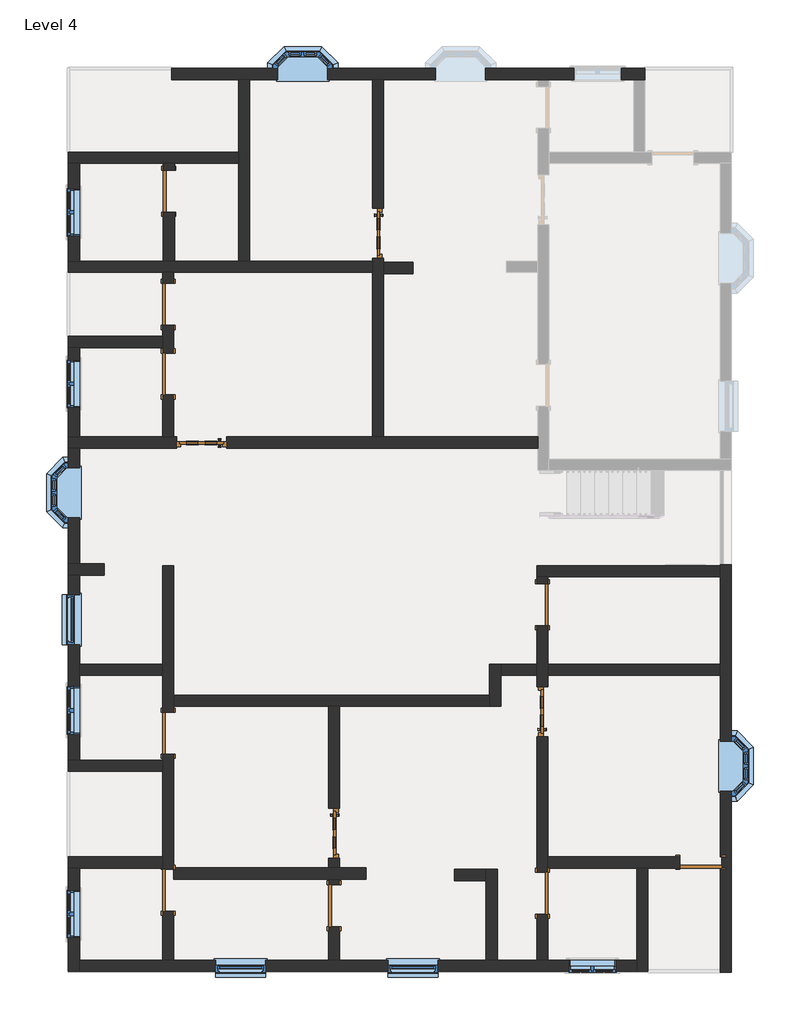
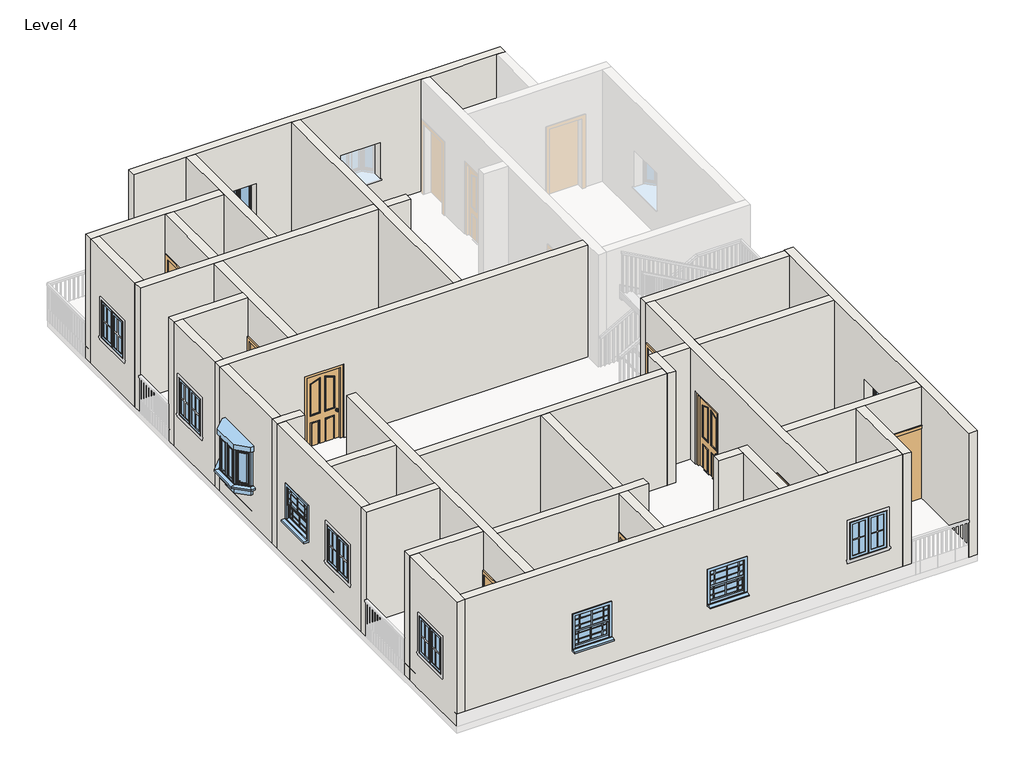
# One storey, part 1 of 4: 34 walls, 13 doors, 11 windows.
"""IFC4 building model written with IfcOpenShell, lengths in millimetres."""

from ifc_helpers import new_model, si_unit, frame, origin, place, context, project, spatial, polyline, outline, extrude, faceted_brep, transform, mapped, element, save
from components import doors_extsgl_12_910x2110mm_9a09825e, door_fadea3f2, door_53b1b562, window_910x910mm_67ef725a, window_c29befe5, windows_sash_w_bars_1_910x910mm_b688f793

model = new_model("IFC4")

# Units and contexts
model_context = context("Model", 3, world=origin())
ifc_project = project(units=[si_unit("LENGTHUNIT", "METRE", prefix="MILLI")], contexts=[model_context])

# Site, building, storey
site = spatial("IfcSite", under=ifc_project)
building = spatial("IfcBuilding", under=site)
storey = spatial("IfcBuildingStorey", under=building, Name="Level 4", Elevation=9144.0)

# Doors
placement = place(None, origin())
doors_extsgl_12_910x2110mm_shape = doors_extsgl_12_910x2110mm_9a09825e(model_context)
element("IfcDoor", 1, ObjectType="Doors_ExtSgl_12 : 910x2110mm", at=placement, inside=storey, context=model_context, shape_type="MappedRepresentation", body=[
    mapped(doors_extsgl_12_910x2110mm_shape, transform((-1409.2058717, 5320.2339901, 9144.0), x_axis=(0.0, -1.0, 0.0), y_axis=(1.0, 0.0, 0.0), z_axis=(0.0, 0.0, 1.0))),
])
element("IfcDoor", 2, ObjectType="Doors_ExtSgl_12 : 910x2110mm", at=placement, inside=storey, context=model_context, shape_type="MappedRepresentation", body=[
    mapped(doors_extsgl_12_910x2110mm_shape, transform((-4622.3058717, 1514.4547293, 9144.0), x_axis=(-1.0, 0.0, 0.0), y_axis=(0.0, -1.0, 0.0), z_axis=(0.0, 0.0, 1.0))),
])
element("IfcDoor", 3, ObjectType="Doors_ExtSgl_12 : 910x2110mm", at=placement, inside=storey, context=model_context, shape_type="MappedRepresentation", body=[
    mapped(doors_extsgl_12_910x2110mm_shape, transform((-2209.3058717, -5597.5452707, 9144.0), x_axis=(0.0, -1.0, 0.0), y_axis=(1.0, 0.0, 0.0), z_axis=(0.0, 0.0, 1.0))),
])
element("IfcDoor", 4, ObjectType="Doors_ExtSgl_12 : 910x2110mm", at=placement, inside=storey, context=model_context, shape_type="MappedRepresentation", body=[
    mapped(doors_extsgl_12_910x2110mm_shape, transform((1587.9941283, -3384.0437545, 9144.0), x_axis=(0.0, 1.0, 0.0), y_axis=(-1.0, 0.0, 0.0), z_axis=(0.0, 0.0, 1.0))),
])
door_shape = door_fadea3f2(model_context)
element("IfcDoor", 5, ObjectType="Single-Flush : 30\" x 80\"", at=placement, inside=storey, context=model_context, shape_type="MappedRepresentation", body=[
    mapped(door_shape, transform((-5219.2058717, 6086.4547293, 9144.0), x_axis=(0.0, 1.0, 0.0), y_axis=(-1.0, 0.0, 0.0), z_axis=(0.0, 0.0, 1.0))),
])
element("IfcDoor", 6, ObjectType="Single-Flush : 30\" x 80\"", at=placement, inside=storey, context=model_context, shape_type="MappedRepresentation", body=[
    mapped(door_shape, transform((-5231.9058717, -6637.2703483, 9144.0), x_axis=(0.0, 1.0, 0.0), y_axis=(-1.0, 0.0, 0.0), z_axis=(0.0, 0.0, 1.0))),
])
element("IfcDoor", 7, ObjectType="Single-Flush : 30\" x 80\"", at=placement, inside=storey, context=model_context, shape_type="MappedRepresentation", body=[
    mapped(door_shape, transform((-2209.3058717, -6918.3452707, 9144.0), x_axis=(0.0, 1.0, 0.0), y_axis=(-1.0, 0.0, 0.0), z_axis=(0.0, 0.0, 1.0))),
])
door_2_shape = door_53b1b562(model_context)
element("IfcDoor", 8, ObjectType="Single-Flush : 30\" x 80\"", at=placement, inside=storey, context=model_context, shape_type="MappedRepresentation", body=[
    mapped(door_2_shape, transform((-5231.9058717, 2759.0547293, 9144.0), x_axis=(0.0, -1.0, 0.0), y_axis=(1.0, 0.0, 0.0), z_axis=(0.0, 0.0, 1.0))),
])
element("IfcDoor", 9, ObjectType="Single-Flush : 30\" x 80\"", at=placement, inside=storey, context=model_context, shape_type="MappedRepresentation", body=[
    mapped(door_2_shape, transform((-5231.9058717, -3778.816952, 9144.0), x_axis=(0.0, -1.0, 0.0), y_axis=(1.0, 0.0, 0.0), z_axis=(0.0, 0.0, 1.0))),
])
element("IfcDoor", 10, ObjectType="Single-Flush : 30\" x 80\"", at=placement, inside=storey, context=model_context, shape_type="MappedRepresentation", body=[
    mapped(door_2_shape, transform((1587.9941283, -6689.7452707, 9144.0), x_axis=(0.0, 1.0, 0.0), y_axis=(-1.0, 0.0, 0.0), z_axis=(0.0, 0.0, 1.0))),
])
element("IfcDoor", 11, ObjectType="Single-Flush : 30\" x 80\"", at=placement, inside=storey, context=model_context, shape_type="MappedRepresentation", body=[
    mapped(door_2_shape, transform((4470.8941283, -6130.9452707, 9144.0), x_axis=(1.0, 0.0, 0.0), y_axis=(0.0, 1.0, 0.0), z_axis=(0.0, 0.0, 1.0))),
])
element("IfcDoor", 12, ObjectType="Single-Flush : 30\" x 80\"", at=placement, inside=storey, context=model_context, shape_type="MappedRepresentation", body=[
    mapped(door_2_shape, transform((1587.9941283, -1440.3867138, 9144.0), x_axis=(0.0, 1.0, 0.0), y_axis=(-1.0, 0.0, 0.0), z_axis=(0.0, 0.0, 1.0))),
])
element("IfcDoor", 13, ObjectType="Single-Flush : 30\" x 80\"", at=placement, inside=storey, context=model_context, shape_type="MappedRepresentation", body=[
    mapped(door_2_shape, transform((-5231.9058717, 4026.9443597, 9144.0), x_axis=(0.0, -1.0, 0.0), y_axis=(1.0, 0.0, 0.0), z_axis=(0.0, 0.0, 1.0))),
])

# Walls
element("IfcWall", 14, ObjectType="Generic - 4.5\"", at=placement, inside=storey, context=model_context, shape_type="Brep", body=[
    faceted_brep([(-1510.8058717, 4865.2339901, 11254.0), (-1510.8058717, 4865.2339901, 9144.0), (-1510.8058717, 4812.2339901, 9144.0), (-1510.8058717, 4609.0339901, 9144.0), (-1510.8058717, 1616.0547293, 9144.0), (-1510.8058717, 1616.0547293, 12192.0), (-1510.8058717, 4609.0339901, 12192.0), (-1510.8058717, 4812.2339901, 12192.0), (-1510.8058717, 8118.4547293, 12192.0), (-1510.8058717, 8118.4547293, 9144.0), (-1510.8058717, 5775.2339901, 9144.0), (-1510.8058717, 5775.2339901, 11254.0), (-1307.6058717, 1616.0547293, 9144.0), (-1307.6058717, 4587.8547293, 9144.0), (-1307.6058717, 4791.0547293, 9144.0), (-1307.6058717, 4865.2339901, 9144.0), (-1307.6058717, 4865.2339901, 11254.0), (-1307.6058717, 5775.2339901, 11254.0), (-1307.6058717, 5775.2339901, 9144.0), (-1307.6058717, 8118.4547293, 9144.0), (-1307.6058717, 8118.4547293, 12192.0), (-1307.6058717, 4791.0547293, 12192.0), (-1307.6058717, 4587.8547293, 12192.0), (-1307.6058717, 1616.0547293, 12192.0)], [[[0, 1, 2, 3, 4, 5, 6, 7, 8, 9, 10, 11]], [[12, 13, 14, 15, 16, 17, 18, 19, 20, 21, 22, 23]], [[10, 9, 19, 18]], [[4, 3, 2, 1, 15, 14, 13, 12]], [[8, 7, 6, 5, 23, 22, 21, 20]], [[9, 8, 20, 19]], [[5, 4, 12, 23]], [[18, 17, 11, 10]], [[16, 15, 1, 0]], [[17, 16, 0, 11]]]),
])
element("IfcWall", 15, ObjectType="Generic - 4.5\"", at=placement, inside=storey, context=model_context, shape_type="Brep", body=[
    faceted_brep([(-7048.0058717, 4609.0339901, 9144.0), (-5333.5058717, 4609.0339901, 9144.0), (-5130.3058717, 4609.0339901, 9144.0), (-1510.8058717, 4609.0339901, 9144.0), (-1510.8058717, 4609.0339901, 12192.0), (-5130.3058717, 4609.0339901, 12192.0), (-5333.5058717, 4609.0339901, 12192.0), (-7048.0058717, 4609.0339901, 12192.0), (-7048.0058717, 4812.2339901, 9144.0), (-7048.0058717, 4812.2339901, 12192.0), (-6844.8058717, 4812.2339901, 12192.0), (-5320.8058717, 4812.2339901, 12192.0), (-5117.6058717, 4812.2339901, 12192.0), (-3949.2058717, 4812.2339901, 12192.0), (-3746.0058717, 4812.2339901, 12192.0), (-1510.8058717, 4812.2339901, 12192.0), (-1510.8058717, 4812.2339901, 9144.0), (-3746.0058717, 4812.2339901, 9144.0), (-3949.2058717, 4812.2339901, 9144.0), (-5117.6058717, 4812.2339901, 9144.0), (-5320.8058717, 4812.2339901, 9144.0), (-6844.8058717, 4812.2339901, 9144.0)], [[[0, 1, 2, 3, 4, 5, 6, 7]], [[8, 9, 10, 11, 12, 13, 14, 15, 16, 17, 18, 19, 20, 21]], [[3, 2, 1, 0, 8, 21, 20, 19, 18, 17, 16]], [[7, 6, 5, 4, 15, 14, 13, 12, 11, 10, 9]], [[4, 3, 16, 15]], [[0, 7, 9, 8]]]),
])
element("IfcWall", 16, ObjectType="Generic - 4.5\"", at=placement, inside=storey, context=model_context, shape_type="Brep", body=[
    faceted_brep([(-3949.2058717, 8118.4547293, 9144.0), (-3949.2058717, 6797.6547293, 9144.0), (-3949.2058717, 6594.4547293, 9144.0), (-3949.2058717, 4812.2339901, 9144.0), (-3949.2058717, 4812.2339901, 12192.0), (-3949.2058717, 6594.4547293, 12192.0), (-3949.2058717, 6797.6547293, 12192.0), (-3949.2058717, 8118.4547293, 12192.0), (-3746.0058717, 8118.4547293, 9144.0), (-3746.0058717, 8118.4547293, 12192.0), (-3746.0058717, 4812.2339901, 12192.0), (-3746.0058717, 4812.2339901, 9144.0)], [[[0, 1, 2, 3, 4, 5, 6, 7]], [[8, 9, 10, 11]], [[3, 2, 1, 0, 8, 11]], [[7, 6, 5, 4, 10, 9]], [[0, 7, 9, 8]], [[4, 3, 11, 10]]]),
])
element("IfcWall", 17, ObjectType="Generic - 4.5\"", at=placement, inside=storey, context=model_context, shape_type="Brep", body=[
    faceted_brep([(-5333.5058717, 3645.9443597, 11176.0), (-5333.5058717, 3645.9443597, 9144.0), (-5333.5058717, 3444.8547293, 9144.0), (-5333.5058717, 3241.6547293, 9144.0), (-5333.5058717, 3140.0547293, 9144.0), (-5333.5058717, 3140.0547293, 11176.0), (-5333.5058717, 2378.0547293, 11176.0), (-5333.5058717, 2378.0547293, 9144.0), (-5333.5058717, 1616.0547293, 9144.0), (-5333.5058717, 1616.0547293, 12192.0), (-5333.5058717, 3241.6547293, 12192.0), (-5333.5058717, 3444.8547293, 12192.0), (-5333.5058717, 4609.0339901, 12192.0), (-5333.5058717, 4609.0339901, 9144.0), (-5333.5058717, 4407.9443597, 9144.0), (-5333.5058717, 4407.9443597, 11176.0), (-5130.3058717, 3140.0547293, 9144.0), (-5130.3058717, 3645.9443597, 9144.0), (-5130.3058717, 3645.9443597, 11176.0), (-5130.3058717, 4407.9443597, 11176.0), (-5130.3058717, 4407.9443597, 9144.0), (-5130.3058717, 4609.0339901, 9144.0), (-5130.3058717, 4609.0339901, 12192.0), (-5130.3058717, 1616.0547293, 12192.0), (-5130.3058717, 1616.0547293, 9144.0), (-5130.3058717, 2378.0547293, 9144.0), (-5130.3058717, 2378.0547293, 11176.0), (-5130.3058717, 3140.0547293, 11176.0)], [[[0, 1, 2, 3, 4, 5, 6, 7, 8, 9, 10, 11, 12, 13, 14, 15]], [[16, 17, 18, 19, 20, 21, 22, 23, 24, 25, 26, 27]], [[8, 7, 25, 24]], [[14, 13, 21, 20]], [[4, 3, 2, 1, 17, 16]], [[12, 11, 10, 9, 23, 22]], [[13, 12, 22, 21]], [[9, 8, 24, 23]], [[26, 25, 7, 6]], [[27, 26, 6, 5]], [[16, 27, 5, 4]], [[18, 17, 1, 0]], [[19, 18, 0, 15]], [[20, 19, 15, 14]]]),
])
element("IfcWall", 18, ObjectType="Generic - 4.5\"", at=placement, inside=storey, context=model_context, shape_type="Brep", body=[
    faceted_brep([(-5130.3058717, -6256.2703483, 11176.0), (-5130.3058717, -6256.2703483, 9144.0), (-5130.3058717, -6230.8703483, 9144.0), (-5130.3058717, -4159.816952, 9144.0), (-5130.3058717, -4159.816952, 11176.0), (-5130.3058717, -3397.816952, 11176.0), (-5130.3058717, -3397.816952, 9144.0), (-5130.3058717, -3286.1452707, 9144.0), (-5130.3058717, -3082.9452707, 9144.0), (-5130.3058717, -733.4452707, 9144.0), (-5130.3058717, -733.4452707, 12192.0), (-5130.3058717, -3082.9452707, 12192.0), (-5130.3058717, -3286.1452707, 12192.0), (-5130.3058717, -6230.8703483, 12192.0), (-5130.3058717, -6434.0703483, 12192.0), (-5130.3058717, -7908.9452707, 12192.0), (-5130.3058717, -7908.9452707, 9144.0), (-5130.3058717, -7018.2703483, 9144.0), (-5130.3058717, -7018.2703483, 11176.0), (-5333.5058717, -4159.816952, 9144.0), (-5333.5058717, -4271.4886333, 9144.0), (-5333.5058717, -4474.6886333, 9144.0), (-5333.5058717, -6029.3452707, 9144.0), (-5333.5058717, -6232.5452707, 9144.0), (-5333.5058717, -6256.2703483, 9144.0), (-5333.5058717, -6256.2703483, 11176.0), (-5333.5058717, -7018.2703483, 11176.0), (-5333.5058717, -7018.2703483, 9144.0), (-5333.5058717, -7908.9452707, 9144.0), (-5333.5058717, -7908.9452707, 12192.0), (-5333.5058717, -6232.5452707, 12192.0), (-5333.5058717, -6029.3452707, 12192.0), (-5333.5058717, -4474.6886333, 12192.0), (-5333.5058717, -4271.4886333, 12192.0), (-5333.5058717, -2727.3452707, 12192.0), (-5333.5058717, -2524.1452707, 12192.0), (-5333.5058717, -733.4452707, 12192.0), (-5333.5058717, -733.4452707, 9144.0), (-5333.5058717, -2524.1452707, 9144.0), (-5333.5058717, -2727.3452707, 9144.0), (-5333.5058717, -3397.816952, 9144.0), (-5333.5058717, -3397.816952, 11176.0), (-5333.5058717, -4159.816952, 11176.0)], [[[0, 1, 2, 3, 4, 5, 6, 7, 8, 9, 10, 11, 12, 13, 14, 15, 16, 17, 18]], [[19, 20, 21, 22, 23, 24, 25, 26, 27, 28, 29, 30, 31, 32, 33, 34, 35, 36, 37, 38, 39, 40, 41, 42]], [[40, 39, 38, 37, 9, 8, 7, 6]], [[17, 16, 28, 27]], [[3, 2, 1, 24, 23, 22, 21, 20, 19]], [[10, 9, 37, 36]], [[15, 14, 13, 12, 11, 10, 36, 35, 34, 33, 32, 31, 30, 29]], [[4, 3, 19, 42]], [[5, 4, 42, 41]], [[6, 5, 41, 40]], [[25, 24, 1, 0]], [[26, 25, 0, 18]], [[27, 26, 18, 17]], [[16, 15, 29, 28]]]),
])
element("IfcWall", 19, ObjectType="Generic - 4.5\"", at=placement, inside=storey, context=model_context, shape_type="Brep", body=[
    faceted_brep([(-7048.0058717, -898.5452707, 9144.0), (-6844.8058717, -898.5452707, 9144.0), (-6400.7404065, -898.5452707, 9144.0), (-6400.7404065, -898.5452707, 12192.0), (-6844.8058717, -898.5452707, 12192.0), (-7048.0058717, -898.5452707, 12192.0), (-7048.0058717, -695.3452707, 9144.0), (-7048.0058717, -695.3452707, 12192.0), (-6844.8058717, -695.3452707, 12192.0), (-6400.7404065, -695.3452707, 12192.0), (-6400.7404065, -695.3452707, 9144.0), (-6844.8058717, -695.3452707, 9144.0)], [[[0, 1, 2, 3, 4, 5]], [[6, 7, 8, 9, 10, 11]], [[2, 1, 0, 6, 11, 10]], [[3, 2, 10, 9]], [[5, 4, 3, 9, 8, 7]], [[0, 5, 7, 6]]]),
])
element("IfcWall", 20, ObjectType="Generic - 4.5\"", at=placement, inside=storey, context=model_context, shape_type="Brep", body=[
    faceted_brep([(-7048.0058717, 6594.4547293, 9144.0), (-6844.8058717, 6594.4547293, 9144.0), (-5320.8058717, 6594.4547293, 9144.0), (-5117.6058717, 6594.4547293, 9144.0), (-3949.2058717, 6594.4547293, 9144.0), (-3949.2058717, 6594.4547293, 12192.0), (-5117.6058717, 6594.4547293, 12192.0), (-5320.8058717, 6594.4547293, 12192.0), (-6844.8058717, 6594.4547293, 12192.0), (-7048.0058717, 6594.4547293, 12192.0), (-7048.0058717, 6797.6547293, 9144.0), (-7048.0058717, 6797.6547293, 12192.0), (-3949.2058717, 6797.6547293, 12192.0), (-3949.2058717, 6797.6547293, 9144.0)], [[[0, 1, 2, 3, 4, 5, 6, 7, 8, 9]], [[10, 11, 12, 13]], [[4, 3, 2, 1, 0, 10, 13]], [[9, 8, 7, 6, 5, 12, 11]], [[5, 4, 13, 12]], [[0, 9, 11, 10]]]),
])
element("IfcWall", 21, ObjectType="Generic - 4.5\"", at=placement, inside=storey, context=model_context, shape_type="Brep", body=[
    faceted_brep([(-7048.0058717, 3241.6547293, 9144.0), (-6844.8058717, 3241.6547293, 9144.0), (-5333.5058717, 3241.6547293, 9144.0), (-5333.5058717, 3241.6547293, 12192.0), (-6844.8058717, 3241.6547293, 12192.0), (-7048.0058717, 3241.6547293, 12192.0), (-7048.0058717, 3444.8547293, 9144.0), (-7048.0058717, 3444.8547293, 12192.0), (-5333.5058717, 3444.8547293, 12192.0), (-5333.5058717, 3444.8547293, 9144.0)], [[[0, 1, 2, 3, 4, 5]], [[6, 7, 8, 9]], [[2, 1, 0, 6, 9]], [[5, 4, 3, 8, 7]], [[3, 2, 9, 8]], [[0, 5, 7, 6]]]),
])
element("IfcWall", 22, ObjectType="Generic - 4.5\"", at=placement, inside=storey, context=model_context, shape_type="Brep", body=[
    faceted_brep([(-7048.0058717, 1412.8547293, 9144.0), (-6844.8058717, 1412.8547293, 9144.0), (-5077.3058717, 1412.8547293, 9144.0), (-5077.3058717, 1412.8547293, 11254.0), (-4167.3058717, 1412.8547293, 11254.0), (-4167.3058717, 1412.8547293, 9144.0), (1499.0941283, 1412.8547293, 9144.0), (1499.0941283, 1412.8547293, 12192.0), (-6844.8058717, 1412.8547293, 12192.0), (-7048.0058717, 1412.8547293, 12192.0), (-5077.3058717, 1616.0547293, 11254.0), (-5077.3058717, 1616.0547293, 9144.0), (-5130.3058717, 1616.0547293, 9144.0), (-5333.5058717, 1616.0547293, 9144.0), (-6844.8058717, 1616.0547293, 9144.0), (-7048.0058717, 1616.0547293, 9144.0), (-7048.0058717, 1616.0547293, 12192.0), (-6844.8058717, 1616.0547293, 12192.0), (-5333.5058717, 1616.0547293, 12192.0), (-5130.3058717, 1616.0547293, 12192.0), (-1510.8058717, 1616.0547293, 12192.0), (-1307.6058717, 1616.0547293, 12192.0), (1499.0941283, 1616.0547293, 12192.0), (1499.0941283, 1616.0547293, 9144.0), (-1307.6058717, 1616.0547293, 9144.0), (-1510.8058717, 1616.0547293, 9144.0), (-4167.3058717, 1616.0547293, 9144.0), (-4167.3058717, 1616.0547293, 11254.0)], [[[0, 1, 2, 3, 4, 5, 6, 7, 8, 9]], [[10, 11, 12, 13, 14, 15, 16, 17, 18, 19, 20, 21, 22, 23, 24, 25, 26, 27]], [[26, 25, 24, 23, 6, 5]], [[15, 14, 13, 12, 11, 2, 1, 0]], [[9, 8, 7, 22, 21, 20, 19, 18, 17, 16]], [[7, 6, 23, 22]], [[5, 4, 27, 26]], [[3, 2, 11, 10]], [[4, 3, 10, 27]], [[0, 9, 16, 15]]]),
])
element("IfcWall", 23, ObjectType="Generic - 4.5\"", at=placement, inside=storey, context=model_context, shape_type="Brep", body=[
    faceted_brep([(1486.3941283, -932.3867138, 9144.0), (1689.5941283, -932.3867138, 9144.0), (4826.4941283, -932.3867138, 9144.0), (4826.4941283, -932.3867138, 12192.0), (1689.5941283, -932.3867138, 12192.0), (1486.3941283, -932.3867138, 12192.0), (1486.3941283, -729.1867138, 9144.0), (1486.3941283, -729.1867138, 12192.0), (4826.4941283, -729.1867138, 12192.0), (4826.4941283, -729.1867138, 9144.0)], [[[0, 1, 2, 3, 4, 5]], [[6, 7, 8, 9]], [[2, 1, 0, 6, 9]], [[5, 4, 3, 8, 7]], [[3, 2, 9, 8]], [[0, 5, 7, 6]]]),
])
element("IfcWall", 24, ObjectType="Generic - 4.5\"", at=placement, inside=storey, context=model_context, shape_type="Brep", body=[
    faceted_brep([(1486.3941283, -932.3867138, 9144.0), (1486.3941283, -1059.3867138, 9144.0), (1486.3941283, -1059.3867138, 11176.0), (1486.3941283, -1821.3867138, 11176.0), (1486.3941283, -1821.3867138, 9144.0), (1486.3941283, -2520.4437545, 9144.0), (1486.3941283, -2723.6437545, 9144.0), (1486.3941283, -2929.0437545, 9144.0), (1486.3941283, -2929.0437545, 11254.0), (1486.3941283, -3839.0437545, 11254.0), (1486.3941283, -3839.0437545, 9144.0), (1486.3941283, -6308.7452707, 9144.0), (1486.3941283, -6308.7452707, 11176.0), (1486.3941283, -7070.7452707, 11176.0), (1486.3941283, -7070.7452707, 9144.0), (1486.3941283, -7908.9452707, 9144.0), (1486.3941283, -7908.9452707, 12192.0), (1486.3941283, -2723.6437545, 12192.0), (1486.3941283, -2520.4437545, 12192.0), (1486.3941283, -932.3867138, 12192.0), (1689.5941283, -1059.3867138, 11176.0), (1689.5941283, -1059.3867138, 9144.0), (1689.5941283, -932.3867138, 9144.0), (1689.5941283, -932.3867138, 12192.0), (1689.5941283, -2520.4437545, 12192.0), (1689.5941283, -2723.6437545, 12192.0), (1689.5941283, -6029.3452707, 12192.0), (1689.5941283, -6232.5452707, 12192.0), (1689.5941283, -7908.9452707, 12192.0), (1689.5941283, -7908.9452707, 9144.0), (1689.5941283, -7070.7452707, 9144.0), (1689.5941283, -7070.7452707, 11176.0), (1689.5941283, -6308.7452707, 11176.0), (1689.5941283, -6308.7452707, 9144.0), (1689.5941283, -6232.5452707, 9144.0), (1689.5941283, -6029.3452707, 9144.0), (1689.5941283, -3839.0437545, 9144.0), (1689.5941283, -3839.0437545, 11254.0), (1689.5941283, -2929.0437545, 11254.0), (1689.5941283, -2929.0437545, 9144.0), (1689.5941283, -2723.6437545, 9144.0), (1689.5941283, -2520.4437545, 9144.0), (1689.5941283, -1821.3867138, 9144.0), (1689.5941283, -1821.3867138, 11176.0)], [[[0, 1, 2, 3, 4, 5, 6, 7, 8, 9, 10, 11, 12, 13, 14, 15, 16, 17, 18, 19]], [[20, 21, 22, 23, 24, 25, 26, 27, 28, 29, 30, 31, 32, 33, 34, 35, 36, 37, 38, 39, 40, 41, 42, 43]], [[30, 29, 15, 14]], [[36, 35, 34, 33, 11, 10]], [[22, 21, 1, 0]], [[42, 41, 40, 39, 7, 6, 5, 4]], [[19, 18, 17, 16, 28, 27, 26, 25, 24, 23]], [[0, 19, 23, 22]], [[10, 9, 37, 36]], [[8, 7, 39, 38]], [[9, 8, 38, 37]], [[12, 11, 33, 32]], [[13, 12, 32, 31]], [[14, 13, 31, 30]], [[2, 1, 21, 20]], [[3, 2, 20, 43]], [[4, 3, 43, 42]], [[16, 15, 29, 28]]]),
])
element("IfcWall", 25, ObjectType="Generic - 4.5\"", at=placement, inside=storey, context=model_context, shape_type="SweptSolid", body=[
    extrude(outline(polyline([(4826.4941283, -2723.6437545), (1689.5941283, -2723.6437545), (1689.5941283, -2520.4437545), (4826.4941283, -2520.4437545), (4826.4941283, -2723.6437545)])), frame((0.0, 0.0, 9144.0), z_axis=(0.0, 0.0, 1.0), x_axis=(1.0, 0.0, 0.0)), (0.0, 0.0, 1.0), 3048.0),
])
element("IfcWall", 26, ObjectType="Generic - 4.5\"", at=placement, inside=storey, context=model_context, shape_type="Brep", body=[
    faceted_brep([(4826.4941283, -6232.5452707, 12192.0), (3505.6941283, -6232.5452707, 12192.0), (3302.4941283, -6232.5452707, 12192.0), (1689.5941283, -6232.5452707, 12192.0), (1689.5941283, -6232.5452707, 9144.0), (3302.4941283, -6232.5452707, 9144.0), (3505.6941283, -6232.5452707, 9144.0), (4089.8941283, -6232.5452707, 9144.0), (4089.8941283, -6232.5452707, 11176.0), (4826.4941283, -6232.5452707, 11176.0), (1689.5941283, -6029.3452707, 12192.0), (4826.4941283, -6029.3452707, 12192.0), (4826.4941283, -6029.3452707, 11176.0), (4089.8941283, -6029.3452707, 11176.0), (4089.8941283, -6029.3452707, 9144.0), (1689.5941283, -6029.3452707, 9144.0)], [[[0, 1, 2, 3, 4, 5, 6, 7, 8, 9]], [[10, 11, 12, 13, 14, 15]], [[4, 15, 14, 7, 6, 5]], [[3, 2, 1, 0, 11, 10]], [[11, 0, 9, 12]], [[4, 3, 10, 15]], [[8, 13, 12, 9]], [[13, 8, 7, 14]]]),
])
element("IfcWall", 27, ObjectType="Generic - 4.5\"", at=placement, inside=storey, context=model_context, shape_type="Brep", body=[
    faceted_brep([(3302.4941283, -6232.5452707, 9144.0), (3302.4941283, -7908.9452707, 9144.0), (3302.4941283, -8112.1452707, 9144.0), (3302.4941283, -8112.1452707, 12192.0), (3302.4941283, -7908.9452707, 12192.0), (3302.4941283, -6232.5452707, 12192.0), (3505.6941283, -6232.5452707, 9144.0), (3505.6941283, -6232.5452707, 12192.0), (3505.6941283, -8112.1452707, 12192.0), (3505.6941283, -8112.1452707, 9144.0)], [[[0, 1, 2, 3, 4, 5]], [[6, 7, 8, 9]], [[2, 1, 0, 6, 9]], [[5, 4, 3, 8, 7]], [[0, 5, 7, 6]], [[3, 2, 9, 8]]]),
])
element("IfcWall", 28, ObjectType="Generic - 4.5\"", at=placement, inside=storey, context=model_context, shape_type="SweptSolid", body=[
    extrude(outline(polyline([(-5333.5058717, -2727.3452707), (-6844.8058717, -2727.3452707), (-6844.8058717, -2524.1452707), (-5333.5058717, -2524.1452707), (-5333.5058717, -2727.3452707)])), frame((0.0, 0.0, 9144.0), z_axis=(0.0, 0.0, 1.0), x_axis=(1.0, 0.0, 0.0)), (0.0, 0.0, 1.0), 3048.0),
])
element("IfcWall", 29, ObjectType="Generic - 4.5\"", at=placement, inside=storey, context=model_context, shape_type="Brep", body=[
    faceted_brep([(-7048.0058717, -4474.6886333, 9144.0), (-5333.5058717, -4474.6886333, 9144.0), (-5333.5058717, -4474.6886333, 12192.0), (-7048.0058717, -4474.6886333, 12192.0), (-7048.0058717, -4271.4886333, 9144.0), (-7048.0058717, -4271.4886333, 12192.0), (-6844.8058717, -4271.4886333, 12192.0), (-5333.5058717, -4271.4886333, 12192.0), (-5333.5058717, -4271.4886333, 9144.0), (-6844.8058717, -4271.4886333, 9144.0)], [[[0, 1, 2, 3]], [[4, 5, 6, 7, 8, 9]], [[1, 0, 4, 9, 8]], [[3, 2, 7, 6, 5]], [[2, 1, 8, 7]], [[0, 3, 5, 4]]]),
])
element("IfcWall", 30, ObjectType="Generic - 4.5\"", at=placement, inside=storey, context=model_context, shape_type="Brep", body=[
    faceted_brep([(-7048.0058717, -6232.5452707, 9144.0), (-6844.8058717, -6232.5452707, 9144.0), (-5333.5058717, -6232.5452707, 9144.0), (-5333.5058717, -6232.5452707, 12192.0), (-6844.8058717, -6232.5452707, 12192.0), (-7048.0058717, -6232.5452707, 12192.0), (-7048.0058717, -6029.3452707, 9144.0), (-7048.0058717, -6029.3452707, 12192.0), (-5333.5058717, -6029.3452707, 12192.0), (-5333.5058717, -6029.3452707, 9144.0)], [[[0, 1, 2, 3, 4, 5]], [[6, 7, 8, 9]], [[2, 1, 0, 6, 9]], [[5, 4, 3, 8, 7]], [[3, 2, 9, 8]], [[0, 5, 7, 6]]]),
])
element("IfcWall", 31, ObjectType="Generic - 4.5\"", at=placement, inside=storey, context=model_context, shape_type="Brep", body=[
    faceted_brep([(-5130.3058717, -6434.0703483, 9144.0), (-2310.9058717, -6434.0703483, 9144.0), (-2107.7058717, -6434.0703483, 9144.0), (-1625.1058717, -6434.0703483, 9144.0), (-1625.1058717, -6434.0703483, 12192.0), (-2107.7058717, -6434.0703483, 12192.0), (-2310.9058717, -6434.0703483, 12192.0), (-5130.3058717, -6434.0703483, 12192.0), (-5130.3058717, -6230.8703483, 9144.0), (-5130.3058717, -6230.8703483, 12192.0), (-2310.9058717, -6230.8703483, 12192.0), (-2107.7058717, -6230.8703483, 12192.0), (-1625.1058717, -6230.8703483, 12192.0), (-1625.1058717, -6230.8703483, 9144.0), (-2107.7058717, -6230.8703483, 9144.0), (-2310.9058717, -6230.8703483, 9144.0), (-5130.3058717, -6256.2703483, 9144.0)], [[[0, 1, 2, 3, 4, 5, 6, 7]], [[8, 9, 10, 11, 12, 13, 14, 15]], [[3, 2, 1, 0, 16, 8, 15, 14, 13]], [[4, 3, 13, 12]], [[7, 6, 5, 4, 12, 11, 10, 9]], [[0, 7, 9, 8, 16]]]),
])
element("IfcWall", 32, ObjectType="Generic - 4.5\"", at=placement, inside=storey, context=model_context, shape_type="Brep", body=[
    faceted_brep([(762.4941283, -7908.9452707, 9144.0), (762.4941283, -6257.9452707, 9144.0), (762.4941283, -6257.9452707, 12192.0), (762.4941283, -7908.9452707, 12192.0), (559.2941283, -7908.9452707, 9144.0), (559.2941283, -7908.9452707, 12192.0), (559.2941283, -6461.1452707, 12192.0), (559.2941283, -6257.9452707, 12192.0), (559.2941283, -6257.9452707, 9144.0), (559.2941283, -6461.1452707, 9144.0)], [[[0, 1, 2, 3]], [[4, 5, 6, 7, 8, 9]], [[1, 0, 4, 9, 8]], [[3, 2, 7, 6, 5]], [[2, 1, 8, 7]], [[0, 3, 5, 4]]]),
])
element("IfcWall", 33, ObjectType="Generic - 4.5\"", at=placement, inside=storey, context=model_context, shape_type="SweptSolid", body=[
    extrude(outline(polyline([(-12.2058717, -6257.9452707), (559.2941283, -6257.9452707), (559.2941283, -6461.1452707), (-12.2058717, -6461.1452707), (-12.2058717, -6257.9452707)])), frame((0.0, 0.0, 9144.0), z_axis=(0.0, 0.0, 1.0), x_axis=(1.0, 0.0, 0.0)), (0.0, 0.0, 1.0), 3048.0),
])
element("IfcWall", 34, ObjectType="Generic - 4.5\"", at=placement, inside=storey, context=model_context, shape_type="SweptSolid", body=[
    extrude(outline(polyline([(-3286.1452707, 12192.0), (-3286.1452707, 9144.0), (-5142.5452707, 9144.0), (-5142.5452707, 11254.0), (-6052.5452707, 11254.0), (-6052.5452707, 9144.0), (-6230.8703483, 9144.0), (-6230.8703483, 12192.0), (-3286.1452707, 12192.0)])), frame((-2310.9058717, 0.0, 0.0), z_axis=(1.0, 0.0, 0.0), x_axis=(0.0, 1.0, 0.0)), (0.0, 0.0, 1.0), 203.2),
    extrude(outline(polyline([(-6537.3452707, 9144.0), (-6537.3452707, 11176.0), (-7299.3452707, 11176.0), (-7299.3452707, 9144.0), (-7908.9452707, 9144.0), (-7908.9452707, 12192.0), (-6434.0703483, 12192.0), (-6434.0703483, 9144.0), (-6537.3452707, 9144.0)])), frame((-2310.9058717, 0.0, 0.0), z_axis=(1.0, 0.0, 0.0), x_axis=(0.0, 1.0, 0.0)), (0.0, 0.0, 1.0), 203.2),
])
element("IfcWall", 35, ObjectType="Generic - 4.5\"", at=placement, inside=storey, context=model_context, shape_type="Brep", body=[
    faceted_brep([(-5130.3058717, -3286.1452707, 9144.0), (-2310.9058717, -3286.1452707, 9144.0), (-2107.7058717, -3286.1452707, 9144.0), (622.0199378, -3286.1452707, 9144.0), (622.0199378, -3286.1452707, 12192.0), (-2107.7058717, -3286.1452707, 12192.0), (-2310.9058717, -3286.1452707, 12192.0), (-5130.3058717, -3286.1452707, 12192.0), (-5130.3058717, -3082.9452707, 9144.0), (-5130.3058717, -3082.9452707, 12192.0), (622.0199378, -3082.9452707, 12192.0), (622.0199378, -3082.9452707, 9144.0)], [[[0, 1, 2, 3, 4, 5, 6, 7]], [[8, 9, 10, 11]], [[3, 2, 1, 0, 8, 11]], [[7, 6, 5, 4, 10, 9]], [[0, 7, 9, 8]], [[4, 3, 11, 10]]]),
])
element("IfcWall", 36, ObjectType="Generic - 4.5\"", at=placement, inside=storey, context=model_context, shape_type="Brep", body=[
    faceted_brep([(825.2199378, -3286.1452707, 9144.0), (825.2199378, -2723.6437545, 9144.0), (825.2199378, -2520.4437545, 9144.0), (825.2199378, -2520.4437545, 12192.0), (825.2199378, -2723.6437545, 12192.0), (825.2199378, -3286.1452707, 12192.0), (622.0199378, -3286.1452707, 9144.0), (622.0199378, -3286.1452707, 12192.0), (622.0199378, -3082.9452707, 12192.0), (622.0199378, -2520.4437545, 12192.0), (622.0199378, -2520.4437545, 9144.0), (622.0199378, -3082.9452707, 9144.0)], [[[0, 1, 2, 3, 4, 5]], [[6, 7, 8, 9, 10, 11]], [[2, 1, 0, 6, 11, 10]], [[5, 4, 3, 9, 8, 7]], [[0, 5, 7, 6]], [[3, 2, 10, 9]]]),
])
element("IfcWall", 37, ObjectType="Generic - 4.5\"", at=placement, inside=storey, context=model_context, shape_type="SweptSolid", body=[
    extrude(outline(polyline([(1486.3941283, -2723.6437545), (825.2199378, -2723.6437545), (825.2199378, -2520.4437545), (1486.3941283, -2520.4437545), (1486.3941283, -2723.6437545)])), frame((0.0, 0.0, 9144.0), z_axis=(0.0, 0.0, 1.0), x_axis=(1.0, 0.0, 0.0)), (0.0, 0.0, 1.0), 3048.0),
])
element("IfcWall", 38, ObjectType="Generic - 4.5\"", at=placement, inside=storey, context=model_context, shape_type="SweptSolid", body=[
    extrude(outline(polyline([(-774.2058717, 4587.8547293), (-1307.6058717, 4587.8547293), (-1307.6058717, 4791.0547293), (-774.2058717, 4791.0547293), (-774.2058717, 4587.8547293)])), frame((0.0, 0.0, 9144.0), z_axis=(0.0, 0.0, 1.0), x_axis=(1.0, 0.0, 0.0)), (0.0, 0.0, 1.0), 3048.0),
])
element("IfcWall", 39, ObjectType="Generic - 4.5\"", at=placement, inside=storey, context=model_context, shape_type="SweptSolid", body=[
    extrude(outline(polyline([(6594.4547293, 9144.0), (6467.4547293, 9144.0), (6467.4547293, 11176.0), (5705.4547293, 11176.0), (5705.4547293, 9144.0), (4812.2339901, 9144.0), (4812.2339901, 12192.0), (6594.4547293, 12192.0), (6594.4547293, 9144.0)])), frame((-5320.8058717, 0.0, 0.0), z_axis=(1.0, 0.0, 0.0), x_axis=(0.0, 1.0, 0.0)), (0.0, 0.0, 1.0), 203.2),
])
element("IfcWall", 40, ObjectType="Generic - 9\"", at=placement, inside=storey, context=model_context, shape_type="Brep", body=[
    faceted_brep([(-5168.4058717, 8118.4547293, 9144.0), (-3949.2058717, 8118.4547293, 9144.0), (-3746.0058717, 8118.4547293, 9144.0), (-1510.8058717, 8118.4547293, 9144.0), (-1307.6058717, 8118.4547293, 9144.0), (1499.0941283, 8118.4547293, 9144.0), (1702.2941283, 8118.4547293, 9144.0), (3251.6941283, 8118.4547293, 9144.0), (3454.8941283, 8118.4547293, 9144.0), (3454.8941283, 8118.4547293, 12192.0), (3251.6941283, 8118.4547293, 12192.0), (1702.2941283, 8118.4547293, 12192.0), (1499.0941283, 8118.4547293, 12192.0), (-1307.6058717, 8118.4547293, 12192.0), (-1510.8058717, 8118.4547293, 12192.0), (-3746.0058717, 8118.4547293, 12192.0), (-3949.2058717, 8118.4547293, 12192.0), (-5168.4058717, 8118.4547293, 12192.0), (-359.2558717, 8118.4547293, 10968.4), (550.7441283, 8118.4547293, 10968.4), (550.7441283, 8118.4547293, 10058.4), (-359.2558717, 8118.4547293, 10058.4), (-3235.8058717, 8118.4547293, 10968.4), (-2325.8058717, 8118.4547293, 10968.4), (-2325.8058717, 8118.4547293, 10058.4), (-3235.8058717, 8118.4547293, 10058.4), (3023.0941283, 8118.4547293, 10972.8), (3023.0941283, 8118.4547293, 10058.4), (2159.4941283, 8118.4547293, 10058.4), (2159.4941283, 8118.4547293, 10972.8), (-5168.4058717, 8321.6547293, 9144.0), (-5168.4058717, 8321.6547293, 12192.0), (3454.8941283, 8321.6547293, 12192.0), (3454.8941283, 8321.6547293, 9144.0), (-359.2558717, 8321.6547293, 10968.4), (-359.2558717, 8321.6547293, 10058.4), (550.7441283, 8321.6547293, 10058.4), (550.7441283, 8321.6547293, 10968.4), (-3235.8058717, 8321.6547293, 10968.4), (-3235.8058717, 8321.6547293, 10058.4), (-2325.8058717, 8321.6547293, 10058.4), (-2325.8058717, 8321.6547293, 10968.4), (3023.0941283, 8321.6547293, 10972.8), (2159.4941283, 8321.6547293, 10972.8), (2159.4941283, 8321.6547293, 10058.4), (3023.0941283, 8321.6547293, 10058.4)], [[[0, 1, 2, 3, 4, 5, 6, 7, 8, 9, 10, 11, 12, 13, 14, 15, 16, 17], [18, 19, 20, 21], [22, 23, 24, 25], [26, 27, 28, 29]], [[30, 31, 32, 33], [34, 35, 36, 37], [38, 39, 40, 41], [42, 43, 44, 45]], [[8, 7, 6, 5, 4, 3, 2, 1, 0, 30, 33]], [[17, 16, 15, 14, 13, 12, 11, 10, 9, 32, 31]], [[0, 17, 31, 30]], [[35, 34, 18, 21]], [[36, 35, 21, 20]], [[37, 36, 20, 19]], [[34, 37, 19, 18]], [[39, 38, 22, 25]], [[40, 39, 25, 24]], [[41, 40, 24, 23]], [[38, 41, 23, 22]], [[27, 26, 42, 45]], [[28, 27, 45, 44]], [[29, 28, 44, 43]], [[26, 29, 43, 42]], [[9, 8, 33, 32]]]),
])
element("IfcWall", 41, ObjectType="Generic - 9\"", at=placement, inside=storey, context=model_context, shape_type="Brep", body=[
    faceted_brep([(4826.4941283, -8124.8452707, 9144.0), (4826.4941283, -8124.8452707, 12192.0), (4826.4941283, -6232.5452707, 12192.0), (4826.4941283, -6029.3452707, 12192.0), (4826.4941283, -2723.6437545, 12192.0), (4826.4941283, -2520.4437545, 12192.0), (4826.4941283, -932.3867138, 12192.0), (4826.4941283, -729.1867138, 12192.0), (4826.4941283, -714.2964201, 12192.0), (4826.4941283, -714.2964201, 9144.0), (4826.4941283, -729.1867138, 9144.0), (4826.4941283, -932.3867138, 9144.0), (4826.4941283, -2520.4437545, 9144.0), (4826.4941283, -2723.6437545, 9144.0), (4826.4941283, -6029.3452707, 9144.0), (4826.4941283, -6029.3452707, 11176.0), (4826.4941283, -6232.5452707, 11176.0), (4826.4941283, -6232.5452707, 9144.0), (4826.4941283, -3921.4945126, 10968.4), (4826.4941283, -4831.4945126, 10968.4), (4826.4941283, -4831.4945126, 10058.4), (4826.4941283, -3921.4945126, 10058.4), (5029.6941283, -8124.8452707, 9144.0), (5029.6941283, -714.2964201, 9144.0), (5029.6941283, -714.2964201, 12192.0), (5029.6941283, -8124.8452707, 12192.0), (5029.6941283, -3921.4945126, 10968.4), (5029.6941283, -3921.4945126, 10058.4), (5029.6941283, -4831.4945126, 10058.4), (5029.6941283, -4831.4945126, 10968.4), (4851.8941283, -6232.5452707, 9144.0), (4851.8941283, -6029.3452707, 9144.0), (4851.8941283, -6232.5452707, 11176.0), (4851.8941283, -6029.3452707, 11176.0)], [[[0, 1, 2, 3, 4, 5, 6, 7, 8, 9, 10, 11, 12, 13, 14, 15, 16, 17], [18, 19, 20, 21]], [[22, 23, 24, 25], [26, 27, 28, 29]], [[23, 22, 0, 17, 30, 31, 14, 13, 12, 11, 10, 9]], [[1, 0, 22, 25]], [[8, 7, 6, 5, 4, 3, 2, 1, 25, 24]], [[9, 8, 24, 23]], [[32, 30, 17, 16]], [[31, 33, 15, 14]], [[33, 32, 16, 15]], [[30, 32, 33, 31]], [[27, 26, 18, 21]], [[28, 27, 21, 20]], [[29, 28, 20, 19]], [[26, 29, 19, 18]]]),
])
element("IfcWall", 42, ObjectType="Generic - 9\"", at=placement, inside=storey, context=model_context, shape_type="SweptSolid", body=[
    extrude(outline(polyline([(6594.4547293, 9144.0), (4812.2339901, 9144.0), (4812.2339901, 12192.0), (6594.4547293, 12192.0), (6594.4547293, 9144.0)]), holes=[polyline([(6135.1443597, 10972.8), (5271.5443597, 10972.8), (5271.5443597, 10058.4), (6135.1443597, 10058.4), (6135.1443597, 10972.8)])]), frame((-7048.0058717, 0.0, 0.0), z_axis=(1.0, 0.0, 0.0), x_axis=(0.0, 1.0, 0.0)), (0.0, 0.0, 1.0), 203.2),
])
element("IfcWall", 43, ObjectType="Generic - 9\"", at=placement, inside=storey, context=model_context, shape_type="SweptSolid", body=[
    extrude(outline(polyline([(3241.6547293, 9144.0), (1616.0547293, 9144.0), (1616.0547293, 12192.0), (3241.6547293, 12192.0), (3241.6547293, 9144.0)]), holes=[polyline([(3013.0547293, 10972.8), (2149.4547293, 10972.8), (2149.4547293, 10058.4), (3013.0547293, 10058.4), (3013.0547293, 10972.8)])]), frame((-7048.0058717, 0.0, 0.0), z_axis=(1.0, 0.0, 0.0), x_axis=(0.0, 1.0, 0.0)), (0.0, 0.0, 1.0), 203.2),
])
element("IfcWall", 44, ObjectType="Generic - 9\"", at=placement, inside=storey, context=model_context, shape_type="Brep", body=[
    faceted_brep([(-7048.0058717, -898.5452707, 9144.0), (-7048.0058717, -4271.4886333, 9144.0), (-7048.0058717, -4271.4886333, 12192.0), (-7048.0058717, -898.5452707, 12192.0), (-7048.0058717, -2166.3452707, 10058.4), (-7048.0058717, -1256.3452707, 10058.4), (-7048.0058717, -1256.3452707, 10968.4), (-7048.0058717, -2166.3452707, 10968.4), (-7048.0058717, -2930.5452707, 10972.8), (-7048.0058717, -3794.1452707, 10972.8), (-7048.0058717, -3794.1452707, 10058.4), (-7048.0058717, -2930.5452707, 10058.4), (-6844.8058717, -898.5452707, 9144.0), (-6844.8058717, -898.5452707, 12192.0), (-6844.8058717, -2524.1452707, 12192.0), (-6844.8058717, -2727.3452707, 12192.0), (-6844.8058717, -4271.4886333, 12192.0), (-6844.8058717, -4271.4886333, 9144.0), (-6844.8058717, -2727.3452707, 9144.0), (-6844.8058717, -2524.1452707, 9144.0), (-6844.8058717, -2166.3452707, 10058.4), (-6844.8058717, -2166.3452707, 10968.4), (-6844.8058717, -1256.3452707, 10968.4), (-6844.8058717, -1256.3452707, 10058.4), (-6844.8058717, -2930.5452707, 10972.8), (-6844.8058717, -2930.5452707, 10058.4), (-6844.8058717, -3794.1452707, 10058.4), (-6844.8058717, -3794.1452707, 10972.8)], [[[0, 1, 2, 3], [4, 5, 6, 7], [8, 9, 10, 11]], [[12, 13, 14, 15, 16, 17, 18, 19], [20, 21, 22, 23], [24, 25, 26, 27]], [[1, 0, 12, 19, 18, 17]], [[3, 2, 16, 15, 14, 13]], [[0, 3, 13, 12]], [[2, 1, 17, 16]], [[21, 20, 4, 7]], [[22, 21, 7, 6]], [[23, 22, 6, 5]], [[20, 23, 5, 4]], [[25, 24, 8, 11]], [[26, 25, 11, 10]], [[27, 26, 10, 9]], [[24, 27, 9, 8]]]),
])
element("IfcWall", 45, ObjectType="Generic - 9\"", at=placement, inside=storey, context=model_context, shape_type="Brep", body=[
    faceted_brep([(-7048.0058717, -6232.5452707, 9144.0), (-7048.0058717, -8112.1452707, 9144.0), (-7048.0058717, -8112.1452707, 12192.0), (-7048.0058717, -6232.5452707, 12192.0), (-7048.0058717, -6638.9452707, 10972.8), (-7048.0058717, -7502.5452707, 10972.8), (-7048.0058717, -7502.5452707, 10058.4), (-7048.0058717, -6638.9452707, 10058.4), (-6844.8058717, -6232.5452707, 9144.0), (-6844.8058717, -6232.5452707, 12192.0), (-6844.8058717, -7908.9452707, 12192.0), (-6844.8058717, -8112.1452707, 12192.0), (-6844.8058717, -8112.1452707, 9144.0), (-6844.8058717, -7908.9452707, 9144.0), (-6844.8058717, -6638.9452707, 10972.8), (-6844.8058717, -6638.9452707, 10058.4), (-6844.8058717, -7502.5452707, 10058.4), (-6844.8058717, -7502.5452707, 10972.8)], [[[0, 1, 2, 3], [4, 5, 6, 7]], [[8, 9, 10, 11, 12, 13], [14, 15, 16, 17]], [[1, 0, 8, 13, 12]], [[3, 2, 11, 10, 9]], [[0, 3, 9, 8]], [[2, 1, 12, 11]], [[15, 14, 4, 7]], [[16, 15, 7, 6]], [[17, 16, 6, 5]], [[14, 17, 5, 4]]]),
])
element("IfcWall", 46, ObjectType="Generic - 9\"", at=placement, inside=storey, context=model_context, shape_type="Brep", body=[
    faceted_brep([(-6844.8058717, -8112.1452707, 9144.0), (3302.4941283, -8112.1452707, 9144.0), (3302.4941283, -8112.1452707, 12192.0), (-6844.8058717, -8112.1452707, 12192.0), (-3456.1058717, -8112.1452707, 10058.4), (-4366.1058717, -8112.1452707, 10058.4), (-4366.1058717, -8112.1452707, 10968.4), (-3456.1058717, -8112.1452707, 10968.4), (-319.2058717, -8112.1452707, 10058.4), (-1229.2058717, -8112.1452707, 10058.4), (-1229.2058717, -8112.1452707, 10968.4), (-319.2058717, -8112.1452707, 10968.4), (2064.2441283, -8112.1452707, 10972.8), (2927.8441283, -8112.1452707, 10972.8), (2927.8441283, -8112.1452707, 10058.4), (2064.2441283, -8112.1452707, 10058.4), (-6844.8058717, -7908.9452707, 9144.0), (-6844.8058717, -7908.9452707, 12192.0), (-5333.5058717, -7908.9452707, 12192.0), (-5130.3058717, -7908.9452707, 12192.0), (-2310.9058717, -7908.9452707, 12192.0), (-2107.7058717, -7908.9452707, 12192.0), (559.2941283, -7908.9452707, 12192.0), (762.4941283, -7908.9452707, 12192.0), (1486.3941283, -7908.9452707, 12192.0), (1689.5941283, -7908.9452707, 12192.0), (3302.4941283, -7908.9452707, 12192.0), (3302.4941283, -7908.9452707, 9144.0), (1689.5941283, -7908.9452707, 9144.0), (1486.3941283, -7908.9452707, 9144.0), (762.4941283, -7908.9452707, 9144.0), (559.2941283, -7908.9452707, 9144.0), (-2107.7058717, -7908.9452707, 9144.0), (-2310.9058717, -7908.9452707, 9144.0), (-5130.3058717, -7908.9452707, 9144.0), (-5333.5058717, -7908.9452707, 9144.0), (-3456.1058717, -7908.9452707, 10058.4), (-3456.1058717, -7908.9452707, 10968.4), (-4366.1058717, -7908.9452707, 10968.4), (-4366.1058717, -7908.9452707, 10058.4), (-319.2058717, -7908.9452707, 10058.4), (-319.2058717, -7908.9452707, 10968.4), (-1229.2058717, -7908.9452707, 10968.4), (-1229.2058717, -7908.9452707, 10058.4), (2064.2441283, -7908.9452707, 10972.8), (2064.2441283, -7908.9452707, 10058.4), (2927.8441283, -7908.9452707, 10058.4), (2927.8441283, -7908.9452707, 10972.8)], [[[0, 1, 2, 3], [4, 5, 6, 7], [8, 9, 10, 11], [12, 13, 14, 15]], [[16, 17, 18, 19, 20, 21, 22, 23, 24, 25, 26, 27, 28, 29, 30, 31, 32, 33, 34, 35], [36, 37, 38, 39], [40, 41, 42, 43], [44, 45, 46, 47]], [[1, 0, 16, 35, 34, 33, 32, 31, 30, 29, 28, 27]], [[3, 2, 26, 25, 24, 23, 22, 21, 20, 19, 18, 17]], [[2, 1, 27, 26]], [[0, 3, 17, 16]], [[37, 36, 4, 7]], [[38, 37, 7, 6]], [[39, 38, 6, 5]], [[36, 39, 5, 4]], [[41, 40, 8, 11]], [[42, 41, 11, 10]], [[43, 42, 10, 9]], [[40, 43, 9, 8]], [[45, 44, 12, 15]], [[46, 45, 15, 14]], [[47, 46, 14, 13]], [[44, 47, 13, 12]]]),
])
element("IfcWall", 47, ObjectType="Generic - 9\"", at=placement, inside=storey, context=model_context, shape_type="SweptSolid", body=[
    extrude(outline(polyline([(1412.8547293, 9144.0), (-695.3452707, 9144.0), (-695.3452707, 12192.0), (1412.8547293, 12192.0), (1412.8547293, 9144.0)]), holes=[polyline([(145.0547293, 10968.4), (145.0547293, 10058.4), (1055.0547293, 10058.4), (1055.0547293, 10968.4), (145.0547293, 10968.4)])]), frame((-7048.0058717, 0.0, 0.0), z_axis=(1.0, 0.0, 0.0), x_axis=(0.0, 1.0, 0.0)), (0.0, 0.0, 1.0), 203.2),
])

# Windows
window_910x910mm_shape = window_910x910mm_67ef725a(model_context)
element("IfcWindow", 48, ObjectType="910x910mm", at=placement, inside=storey, context=model_context, shape_type="MappedRepresentation", body=[
    mapped(window_910x910mm_shape, transform((4919.6375605, -4946.4945126, 8858.4), x_axis=(0.0, -1.0, 0.0), y_axis=(1.0, 0.0, 0.0), z_axis=(0.0, 0.0, 1.0))),
])
element("IfcWindow", 49, ObjectType="910x910mm", at=placement, inside=storey, context=model_context, shape_type="MappedRepresentation", body=[
    mapped(window_910x910mm_shape, transform((-2210.8058717, 8211.5981615, 8858.4), x_axis=(1.0, 0.0, 0.0), y_axis=(0.0, 1.0, 0.0), z_axis=(0.0, 0.0, 1.0))),
])
element("IfcWindow", 50, ObjectType="910x910mm", at=placement, inside=storey, context=model_context, shape_type="MappedRepresentation", body=[
    mapped(window_910x910mm_shape, transform((-6937.9493039, 1170.0547293, 8858.4), x_axis=(0.0, 1.0, 0.0), y_axis=(-1.0, 0.0, 0.0), z_axis=(0.0, 0.0, 1.0))),
])
window_shape = window_c29befe5(model_context)
element("IfcWindow", 51, ObjectType="Window-Casement-Double : 34\" x 36\"", at=placement, inside=storey, context=model_context, shape_type="MappedRepresentation", body=[
    mapped(window_shape, transform((-6946.4058717, 5703.3443597, 9144.0), x_axis=(0.0, 1.0, 0.0), y_axis=(-1.0, 0.0, 0.0), z_axis=(0.0, 0.0, 1.0))),
])
element("IfcWindow", 52, ObjectType="Window-Casement-Double : 34\" x 36\"", at=placement, inside=storey, context=model_context, shape_type="MappedRepresentation", body=[
    mapped(window_shape, transform((-6946.4058717, 2581.2547293, 9144.0), x_axis=(0.0, 1.0, 0.0), y_axis=(-1.0, 0.0, 0.0), z_axis=(0.0, 0.0, 1.0))),
])
element("IfcWindow", 53, ObjectType="Window-Casement-Double : 34\" x 36\"", at=placement, inside=storey, context=model_context, shape_type="MappedRepresentation", body=[
    mapped(window_shape, transform((2496.0441283, -8010.5452707, 9144.0), x_axis=(-1.0, 0.0, 0.0), y_axis=(0.0, -1.0, 0.0), z_axis=(0.0, 0.0, 1.0))),
])
element("IfcWindow", 54, ObjectType="Window-Casement-Double : 34\" x 36\"", at=placement, inside=storey, context=model_context, shape_type="MappedRepresentation", body=[
    mapped(window_shape, transform((-6946.4058717, -7070.7452707, 9144.0), x_axis=(0.0, 1.0, 0.0), y_axis=(-1.0, 0.0, 0.0), z_axis=(0.0, 0.0, 1.0))),
])
element("IfcWindow", 55, ObjectType="Window-Casement-Double : 34\" x 36\"", at=placement, inside=storey, context=model_context, shape_type="MappedRepresentation", body=[
    mapped(window_shape, transform((-6946.4058717, -3362.3452707, 9144.0), x_axis=(0.0, 1.0, 0.0), y_axis=(-1.0, 0.0, 0.0), z_axis=(0.0, 0.0, 1.0))),
])
windows_sash_w_bars_1_910x910mm_shape = windows_sash_w_bars_1_910x910mm_b688f793(model_context)
element("IfcWindow", 56, ObjectType="Windows_Sash_w-Bars_1 : 910x910mm", at=placement, inside=storey, context=model_context, shape_type="MappedRepresentation", body=[
    mapped(windows_sash_w_bars_1_910x910mm_shape, transform((-3911.1058717, -8010.5452707, 9258.4), x_axis=(-1.0, 0.0, 0.0), y_axis=(0.0, -1.0, 0.0), z_axis=(0.0, 0.0, 1.0))),
])
element("IfcWindow", 57, ObjectType="Windows_Sash_w-Bars_1 : 910x910mm", at=placement, inside=storey, context=model_context, shape_type="MappedRepresentation", body=[
    mapped(windows_sash_w_bars_1_910x910mm_shape, transform((-6946.4058717, -1711.3452707, 9258.4), x_axis=(0.0, 1.0, 0.0), y_axis=(-1.0, 0.0, 0.0), z_axis=(0.0, 0.0, 1.0))),
])
element("IfcWindow", 58, ObjectType="Windows_Sash_w-Bars_1 : 910x910mm", at=placement, inside=storey, context=model_context, shape_type="MappedRepresentation", body=[
    mapped(windows_sash_w_bars_1_910x910mm_shape, transform((-774.2058717, -8010.5452707, 9258.4), x_axis=(-1.0, 0.0, 0.0), y_axis=(0.0, -1.0, 0.0), z_axis=(0.0, 0.0, 1.0))),
])

save(model, "model.ifc")

# Revit data of these elements
# Type "Doors_ExtSgl_12 : 910x2110mm"
#   Type Mark = "10"
#   Type Comments = "External Single"
#   Operation = "SingleSwingRight"
#   Construction Type Id = "SGL"
#   Keynote = "L20"
#   Analytic Construction = "Large single-glazed windows"
#   Wrap Layers (Int) from Ext = 0' - 6.98819"
#   Wrap Layers (Ext) from Ext = 0' - 4.03543"
#   Visual Light Transmittance = 0.9
#   Thickness = 0' - 1.73228"
#   Stile Top of Lock rail = 3' - 3.37008"
#   Stile Top Rail = 0' - 5.90551"
#   Stile Shutting = 0' - 4.92126"
#   Stile Muntin Rail = 0' - 4.92126"
#   Stile Lock Rail = 0' - 6.88976"
#   Stile Hanging = 0' - 4.92126"
#   Stile Bottom Rail = 0' - 6.88976"
#   Solar Heat Gain Coefficient = 0.86
#   Rough Width = 2' - 11.82677"
#   Rough Height = 6' - 11.07087"
#   O/A Frame Width = 0' - 2.51969"
#   Heat Transfer Coefficient (U) = 0.979472 BTU/(h·ft²·°F)
#   Handle Z Distance = 3' - 3.37008"
#   Glazing Thickness = 0' - 0.94488"
#   FrameWidth = 0' - 1.65354"
#   FrameOffset - External = 0' - 0.98425"
#   FrameDepth = 0' - 3.50394"
#   Door Panel Width = 2' - 7.77165"
#   Door Panel Thickness = 0' - 1.73228"
#   Door Panel Height = 6' - 6.74016"
#   Cill Thickness = 0' - 2.14567"
#   Cill Projection = 0' - 1.1811"
#   Handle X Distance = 0' - 2.95276"
#   Height = 6' - 11.07087"
#   Structural Tolerance = 0' - 0.25591"
#   Tolerance = 0' - 0.11811"
#   Undercut = 0' - 0.15748"
#   Width = 2' - 11.82677"
#   Cill Extension = 0' - 0.98425"
#   Cavity Closer Width = 0' - 1.9685"
#   Cavity Closer Offset from Ext = 0' - 4.03543"
#   Cavity Closer Depth = 0' - 3.34646"
#   Vis - Ironmongery = yes
#   Vis - Cavity Closers = yes
#   Define Thermal Properties by = 1
#   Function = 1
#   Material Glass = Door - Glazing
#   Material Door = Door - Panel
#   Material Frame = Door - Frame/Mullion
#   Material Ironmongery = Door - Handle
#   Wall Closure = (empty or 0)
# Type "Single-Flush : 30\" x 80\""
#   Type Mark = "5"
#   Construction Type Id = "MDOOR"
#   Assembly Code = "C1020"
#   Analytic Construction = "Metal"
#   Thickness = 0' - 2"
#   Heat Transfer Coefficient (U) = 0.651978 BTU/(h·ft²·°F)
#   Height = 6' - 8"
#   Trim Projection Ext = 0' - 1"
#   Trim Projection Int = 0' - 1"
#   Trim Width = 0' - 3"
#   Width = 2' - 6"
#   Define Thermal Properties by = 1
#   Define Thermal Properties by = 1
#   Door Material = Door - Panel
#   Frame Material = Door - Frame
#   Visual Light Transmittance = 0
#   Solar Heat Gain Coefficient = 0
#   Function = (empty or 0)
#   Wall Closure = (empty or 0)
# Type "Generic - 4.5\""
#   Assembly Code = "B2010"
#   Layers, outside or top first: 0' - 8" no material (function 1)
# Type "Generic - 9\""
#   Assembly Code = "B2010"
#   Layers, outside or top first: 0' - 8" no material (function 1)
# Type "910x910mm"
#   Type Mark = "18"
#   Operation = "UserDefined"
#   Construction Type Id = "GSP4R"
#   Keynote = "L10"
#   Analytic Construction = "1/8 in Pilkington single glazing"
#   Wrap Layers (Ext) from Ext = 0' - 4.03543"
#   Wrap Layers (Int) from Ext = 0' - 6.98819"
#   Window Board Projection = 0' - 0.98425"
#   Window Board Extention = 0' - 0.98425"
#   Visual Light Transmittance = 0.9
#   Solar Heat Gain Coefficient = 0.78
#   Heat Transfer Coefficient (U) = 0.6496 BTU/(h·ft²·°F)
#   Glazing Thickness = 0' - 0.94488"
#   DONT CHANGE - Splay Width = 0' - 7.41997"
#   Rough Width = 2' - 11.82677"
#   Rough Height = 2' - 11.82677"
#   Roof Thickness = 0' - 4.92126"
#   Roof Overhang = 0' - 1.5748"
#   Plinth Thickness = 0' - 6.88976"
#   Height = 2' - 11.82677"
#   Width = 2' - 11.82677"
#   Frame Depth = 0' - 2.55906"
#   Default Head Height = 6' - 11.07087"
#   Cill Depth = 0' - 3.44488"
#   Cavity Closer Width = 0' - 1.9685"
#   Cavity Closer Offset from Ext = 0' - 4.03543"
#   Cavity Closer Depth = 0' - 3.34646"
#   Vis - Cavity Closers = yes
#   Define Thermal Properties by = 1
#   Material Trim = Window Frame
#   Material Glass = Glass
#   Material Frame = Window Frame
#   Manufacturer = ""
#   Wall Closure = (empty or 0)
# Type "Window-Casement-Double : 34\" x 36\""
#   Type Mark = "14"
#   Fire Rating = "0.5h"
#   Assembly Code = "B2020100"
#   Analytic Construction = "Double glazing - domestic"
#   Frame Extension [instance default] = 0' - 0 1/4"
#   Window Inset [instance default] = 0' - 0"
#   Wall Thickness [instance default] = 0' - 6"
#   Interior Wall Closure [instance default] = 0' - 2 1/4"
#   Half Width = 1' - 5"
#   Visual Light Transmittance = 0.81
#   Thermal Resistance (R) = 1.8146 (h·ft²·°F)/BTU
#   Solar Heat Gain Coefficient = 0.76
#   Rough Width = 2' - 10 1/2"
#   Rough Height = 3' - 0 1/2"
#   Height = 3' - 0"
#   Heat Transfer Coefficient (U) = 0.5511 BTU/(h·ft²·°F)
#   Exterior Wall Closure [instance default] = 0' - 1 1/4"
#   Extension Jamb [instance default] = 0' - 2 1/4"
#   Default Sill Height = 3' - 0"
#   Width = 2' - 10"
#   Define Thermal Properties by = 0
#   Muntin Visibility = yes
#   Interior Trim Visibility [instance default] = yes
#   Exterior Trim Visibility [instance default] = yes
#   Extension Jamb Visibility [instance default] = yes
#   Interior Trim Material = Wood - Stained
#   Muntin Pattern = Muntin Pattern_2x2 : Muntin Pattern_2x2
#   Interior Trim = Trim-Window-Interior-Flat : Picture Frame
#   Interior Frame Material = Wood - Stained
#   Glass Panel Material = Glass
#   Exterior Trim Material = Clad - White
#   Exterior Trim = Trim-Window-Exterior-Flat : with Sill
#   Exterior Frame Material = Clad - White
#   Wall Closure = (empty or 0)
# Type "Windows_Sash_w-Bars_1 : 910x910mm"
#   Type Mark = "24"
#   Construction Type Id = "GSP4R"
#   Analytic Construction = "1/8 in Pilkington single glazing"
#   Wrap Layers (Int) from Ext = 0' - 6.98819"
#   Wrap Layers (Ext) from Ext = 0' - 4.03543"
#   Window Board Projection = 0' - 0.98425"
#   Window Board Extension = 0' - 0.98425"
#   Visual Light Transmittance = 0.9
#   Solar Heat Gain Coefficient = 0.78
#   Rough Width = 2' - 11.82677"
#   Rough Height = 2' - 11.82677"
#   Height = 2' - 11.82677"
#   Heat Transfer Coefficient (U) = 0.6496 BTU/(h·ft²·°F)
#   Glazing Thickness = 0' - 0.94488"
#   Glazing Bar Offset = 0' - 3.93701"
#   Frame Depth = 0' - 3.54331"
#   FrameOffset - External = 0' - 1.9685"
#   Default Sill Height = 2' - 7.49606"
#   Width = 2' - 11.82677"
#   Glazing Bar Thickness = 0' - 0.7874"
#   Cavity Closer Width = 0' - 1.9685"
#   Cavity Closer Offset from Ext = 0' - 4.03543"
#   Cavity Closer Depth = 0' - 3.34646"
#   Vis - Vert Bar Top = yes
#   Vis - Vert Bar Bttm = yes
#   Vis - Glazing Bars Top = yes
#   Vis - Glazing Bars Bttm = yes
#   Vis - Cavity Closers = yes
#   Define Thermal Properties by = 1
#   Material Trim = Window Frame
#   Material Frame = Window Frame
#   Material Glazing Bars = Window Frame
#   Material Glass = Glass
#   Wall Closure = (empty or 0)
# Elements 1, 2, 3, 4 (IfcDoor, "Doors_ExtSgl_12 : 910x2110mm")
#   Phase Created = New Construction
#   Materials on its faces: "Door - Panel", "Door - Handle", "Door - Frame/Mullion", "Door - Glazing"
# Elements 5, 6, 7, 8, 9, 10, 11, 12, 13 (IfcDoor, "Single-Flush : 30\" x 80\"")
#   Phase Created = New Construction
